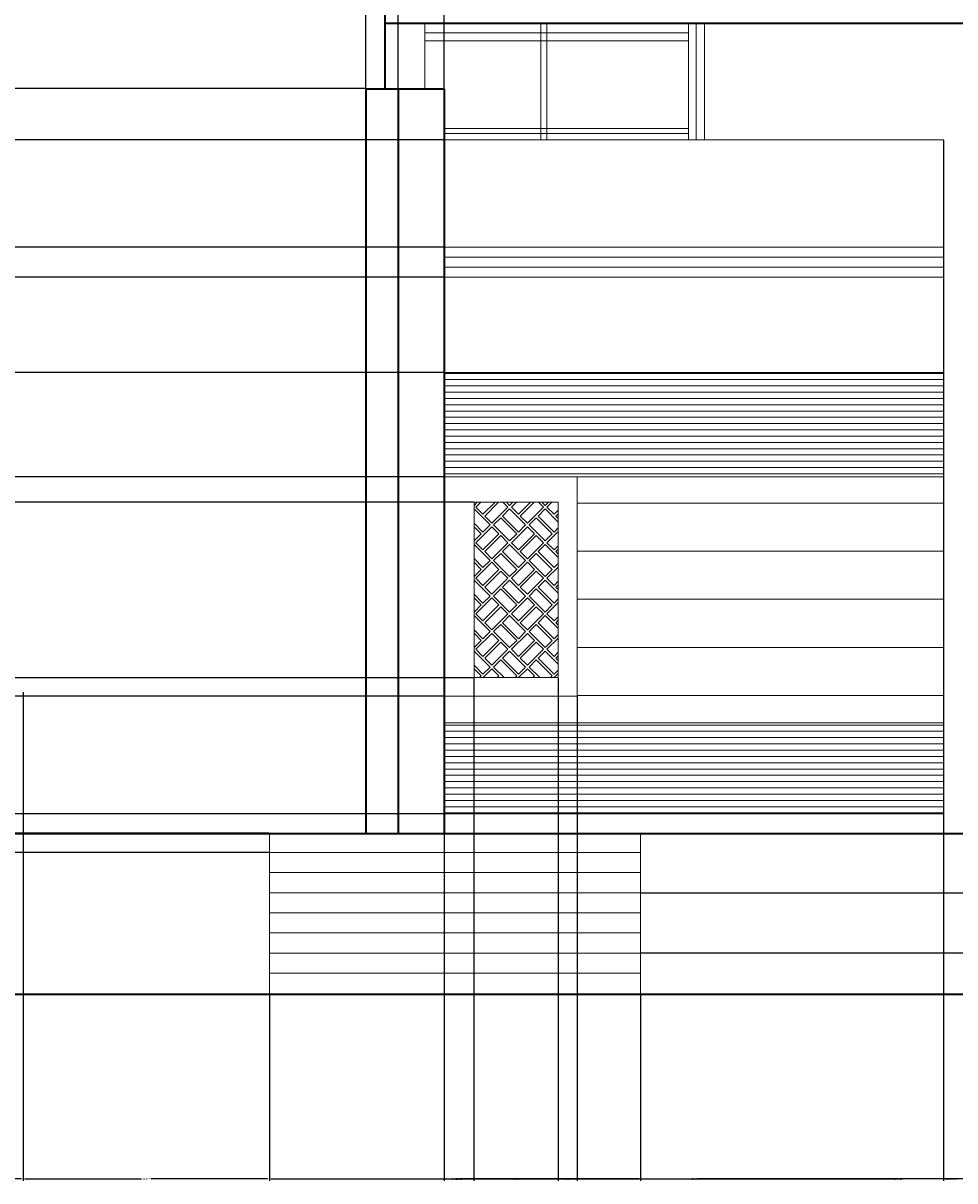
# Model space of a CAD drawing. Units: inches. Extents: x -7 to 391, y -12 to 303.
# Tile 3 of 5: x 222 to 315, y -12 to 103. Entities that reach past the tile are written whole.
import ezdxf

# ---------------------------------------------------------------- set-up
doc = ezdxf.new("R2010")
doc.units = ezdxf.units.IN
doc.header["$MEASUREMENT"] = 0
for name, color, linetype, lineweight in [('A-ANNO-DIMS', 2, 'Continuous', 18), ('A-DOOR', 3, 'Continuous', 18), ('A-ELEV', 7, 'Continuous', 35), ('A-ELEV-PATT', 8, 'Continuous', 13), ('A-FLOR-STRS', 2, 'Continuous', 18), ('A-GLAZ', 4, 'Continuous', 18)]:
    doc.layers.add(name, color=color, linetype=linetype, lineweight=lineweight)
doc.styles.get("Standard").update_dxf_attribs({"font": 'arial.ttf'})
doc.dimstyles.get("Standard").update_dxf_attribs({"dimtxt": 0.18, "dimasz": 0.18, "dimexe": 0.18, "dimexo": 0.0625, "dimgap": 0.09, "dimtad": 0, "dimtih": 1, "dimtoh": 1, "dimdec": 4, "dimzin": 0, "dimdsep": 46, "dimtxsty": 'Standard', "dimcen": 0.09, "dimadec": 0, "dimazin": 0, "dimtfac": 1, "dimtdec": 4, "dimtofl": 0, "dimtmove": 0, "dimatfit": 3, "dimfxl": 1, "dimtolj": 1, "dimtzin": 0, "dimarcsym": 0})

# ---------------------------------------------------------------- blocks, each defined once
blk = doc.blocks.new('*D1')
at = {"layer": 'A-ANNO-DIMS', "color": 0, "lineweight": -2, "transparency": 16777216}
for p, q in [((372.08, 122.18), (390.6, 122.18)), ((390.42, 122), (390.42, 64.44)), ((390.42, 6.53), (390.42, 64.08)), ((150.31, 6.35), (390.6, 6.35))]:
    blk.add_line(p, q, dxfattribs=at)
at = {"layer": 'A-ANNO-DIMS', "color": 0, "transparency": 16777216}
for points in [[(390.39, 122), (390.45, 122), (390.42, 122.18)], [(390.39, 6.53), (390.45, 6.53), (390.42, 6.35)]]:
    blk.add_solid(points, dxfattribs=at)
at = {"layer": 'Defpoints', "color": 0, "transparency": 16777216}
for p in [(372.02, 122.18), (390.42, 122.18), (150.24, 6.35)]:
    blk.add_point(p, dxfattribs=at)
at = {"layer": 'A-ANNO-DIMS', "color": 0, "transparency": 16777216, "insert": (390.42, 64.26), "char_height": 0.18, "attachment_point": 5}
blk.add_mtext('\\A1;115.83', dxfattribs=at)
blk = doc.blocks.new('*D37')
at = {"layer": 'A-ANNO-DIMS', "color": 0, "lineweight": -2, "transparency": 16777216}
for p, q in [((207.51, 38.39), (207.51, -12.23)), ((222.24, 36.39), (222.24, -12.23)), ((207.69, -12.05), (214.42, -12.05)), ((222.06, -12.05), (215.33, -12.05))]:
    blk.add_line(p, q, dxfattribs=at)
at = {"layer": 'A-ANNO-DIMS', "color": 0, "transparency": 16777216}
for points in [[(207.69, -12.02), (207.69, -12.08), (207.51, -12.05)], [(222.06, -12.02), (222.06, -12.08), (222.24, -12.05)]]:
    blk.add_solid(points, dxfattribs=at)
at = {"layer": 'Defpoints', "color": 0, "transparency": 16777216}
for p in [(207.51, 38.46), (222.24, 36.46), (222.24, -12.05)]:
    blk.add_point(p, dxfattribs=at)
at = {"layer": 'A-ANNO-DIMS', "color": 0, "transparency": 16777216, "insert": (214.88, -12.05), "char_height": 0.18, "attachment_point": 5}
blk.add_mtext('\\A1;14.734', dxfattribs=at)
blk = doc.blocks.new('*D38')
at = {"layer": 'A-ANNO-DIMS', "color": 0, "lineweight": -2, "transparency": 16777216}
for p, q in [((222.24, 36.39), (222.24, -12.23)), ((246.74, 6.28), (246.74, -12.23)), ((222.42, -12.05), (234.03, -12.05)), ((246.56, -12.05), (234.96, -12.05))]:
    blk.add_line(p, q, dxfattribs=at)
at = {"layer": 'A-ANNO-DIMS', "color": 0, "transparency": 16777216}
for points in [[(222.42, -12.02), (222.42, -12.08), (222.24, -12.05)], [(246.56, -12.02), (246.56, -12.08), (246.74, -12.05)]]:
    blk.add_solid(points, dxfattribs=at)
at = {"layer": 'Defpoints', "color": 0, "transparency": 16777216}
for p in [(222.24, 36.46), (246.74, 6.35), (246.74, -12.05)]:
    blk.add_point(p, dxfattribs=at)
at = {"layer": 'A-ANNO-DIMS', "color": 0, "transparency": 16777216, "insert": (234.49, -12.05), "char_height": 0.18, "attachment_point": 5}
blk.add_mtext('\\A1;24.497', dxfattribs=at)
blk = doc.blocks.new('*D39')
at = {"layer": 'A-ANNO-DIMS', "color": 0, "lineweight": -2, "transparency": 16777216}
for p, q in [((372.02, 154.28), (372.02, -12.23)), ((246.74, 6.28), (246.74, -12.23)), ((246.92, -12.05), (308.92, -12.05)), ((371.84, -12.05), (309.84, -12.05))]:
    blk.add_line(p, q, dxfattribs=at)
at = {"layer": 'A-ANNO-DIMS', "color": 0, "transparency": 16777216}
for points in [[(246.92, -12.02), (246.92, -12.08), (246.74, -12.05)], [(371.84, -12.02), (371.84, -12.08), (372.02, -12.05)]]:
    blk.add_solid(points, dxfattribs=at)
at = {"layer": 'Defpoints', "color": 0, "transparency": 16777216}
for p in [(372.02, 154.35), (246.74, 6.35), (372.02, -12.05)]:
    blk.add_point(p, dxfattribs=at)
at = {"layer": 'A-ANNO-DIMS', "color": 0, "transparency": 16777216, "insert": (309.38, -12.05), "char_height": 0.18, "attachment_point": 5}
blk.add_mtext('\\A1;125.28', dxfattribs=at)
blk = doc.blocks.new('*D40')
at = {"layer": 'A-ANNO-DIMS', "color": 0, "lineweight": -2, "transparency": 16777216}
for p, q in [((246.74, 6.28), (246.74, -12.23)), ((283.68, 6.28), (283.68, -12.23)), ((246.92, -12.05), (264.82, -12.05)), ((283.5, -12.05), (265.6, -12.05))]:
    blk.add_line(p, q, dxfattribs=at)
at = {"layer": 'A-ANNO-DIMS', "color": 0, "transparency": 16777216}
for points in [[(246.92, -12.02), (246.92, -12.08), (246.74, -12.05)], [(283.5, -12.02), (283.5, -12.08), (283.68, -12.05)]]:
    blk.add_solid(points, dxfattribs=at)
at = {"layer": 'Defpoints', "color": 0, "transparency": 16777216}
for p in [(246.74, 6.35), (283.68, 6.35), (283.68, -12.05)]:
    blk.add_point(p, dxfattribs=at)
at = {"layer": 'A-ANNO-DIMS', "color": 0, "transparency": 16777216, "insert": (265.21, -12.05), "char_height": 0.18, "attachment_point": 5}
blk.add_mtext('\\A1;36.94', dxfattribs=at)
blk = doc.blocks.new('*D41')
at = {"layer": 'A-ANNO-DIMS', "color": 0, "lineweight": -2, "transparency": 16777216}
for p, q in [((283.68, 6.28), (283.68, -12.23)), ((335.08, 6.28), (335.08, -12.23)), ((283.86, -12.05), (309.06, -12.05)), ((334.9, -12.05), (309.7, -12.05))]:
    blk.add_line(p, q, dxfattribs=at)
at = {"layer": 'A-ANNO-DIMS', "color": 0, "transparency": 16777216}
for points in [[(283.86, -12.02), (283.86, -12.08), (283.68, -12.05)], [(334.9, -12.02), (334.9, -12.08), (335.08, -12.05)]]:
    blk.add_solid(points, dxfattribs=at)
at = {"layer": 'Defpoints', "color": 0, "transparency": 16777216}
for p in [(283.68, 6.35), (335.08, 6.35), (335.08, -12.05)]:
    blk.add_point(p, dxfattribs=at)
at = {"layer": 'A-ANNO-DIMS', "color": 0, "transparency": 16777216, "insert": (309.38, -12.05), "char_height": 0.18, "attachment_point": 5}
blk.add_mtext('\\A1;51.4', dxfattribs=at)
blk = doc.blocks.new('*D43')
at = {"layer": 'A-ANNO-DIMS', "color": 0, "lineweight": -2, "transparency": 16777216}
for p, q in [((267.1, 37.78), (267.1, -12.23)), ((264.13, 35.95), (264.13, -12.23)), ((264.31, -12.05), (265.24, -12.05)), ((266.92, -12.05), (266, -12.05))]:
    blk.add_line(p, q, dxfattribs=at)
at = {"layer": 'A-ANNO-DIMS', "color": 0, "transparency": 16777216}
for points in [[(264.31, -12.02), (264.31, -12.08), (264.13, -12.05)], [(266.92, -12.02), (266.92, -12.08), (267.1, -12.05)]]:
    blk.add_solid(points, dxfattribs=at)
at = {"layer": 'Defpoints', "color": 0, "transparency": 16777216}
for p in [(267.1, 37.84), (264.13, 36.01), (267.1, -12.05)]:
    blk.add_point(p, dxfattribs=at)
at = {"layer": 'A-ANNO-DIMS', "color": 0, "transparency": 16777216, "insert": (265.62, -12.05), "char_height": 0.18, "attachment_point": 5}
blk.add_mtext('\\A1;2.971', dxfattribs=at)
blk = doc.blocks.new('*D44')
at = {"layer": 'A-ANNO-DIMS', "color": 0, "lineweight": -2, "transparency": 16777216}
for p, q in [((267.1, 37.78), (267.1, -12.23)), ((275.48, 37.78), (275.48, -12.23)), ((267.28, -12.05), (270.9, -12.05)), ((275.3, -12.05), (271.69, -12.05))]:
    blk.add_line(p, q, dxfattribs=at)
at = {"layer": 'A-ANNO-DIMS', "color": 0, "transparency": 16777216}
for points in [[(267.28, -12.02), (267.28, -12.08), (267.1, -12.05)], [(275.3, -12.02), (275.3, -12.08), (275.48, -12.05)]]:
    blk.add_solid(points, dxfattribs=at)
at = {"layer": 'Defpoints', "color": 0, "transparency": 16777216}
for p in [(267.1, 37.84), (275.48, 37.84), (275.48, -12.05)]:
    blk.add_point(p, dxfattribs=at)
at = {"layer": 'A-ANNO-DIMS', "color": 0, "transparency": 16777216, "insert": (271.29, -12.05), "char_height": 0.18, "attachment_point": 5}
blk.add_mtext('\\A1;8.377', dxfattribs=at)
blk = doc.blocks.new('*D45')
at = {"layer": 'A-ANNO-DIMS', "color": 0, "lineweight": -2, "transparency": 16777216}
for p, q in [((275.48, 37.78), (275.48, -12.23)), ((277.36, 35.95), (277.36, -12.23)), ((275.66, -12.05), (276.1, -12.05)), ((277.18, -12.05), (276.74, -12.05))]:
    blk.add_line(p, q, dxfattribs=at)
at = {"layer": 'A-ANNO-DIMS', "color": 0, "transparency": 16777216}
for points in [[(275.66, -12.02), (275.66, -12.08), (275.48, -12.05)], [(277.18, -12.02), (277.18, -12.08), (277.36, -12.05)]]:
    blk.add_solid(points, dxfattribs=at)
at = {"layer": 'Defpoints', "color": 0, "transparency": 16777216}
for p in [(275.48, 37.84), (277.36, 36.01), (277.36, -12.05)]:
    blk.add_point(p, dxfattribs=at)
at = {"layer": 'A-ANNO-DIMS', "color": 0, "transparency": 16777216, "insert": (276.42, -12.05), "char_height": 0.18, "attachment_point": 5}
blk.add_mtext('\\A1;1.88', dxfattribs=at)
blk = doc.blocks.new('*D46')
at = {"layer": 'A-ANNO-DIMS', "color": 0, "lineweight": -2, "transparency": 16777216}
for p, q in [((256.34, 96.52), (256.34, 303.01)), ((259.55, 96.52), (259.55, 303.01)), ((256.52, 302.83), (257.55, 302.83)), ((259.37, 302.83), (258.34, 302.83))]:
    blk.add_line(p, q, dxfattribs=at)
at = {"layer": 'A-ANNO-DIMS', "color": 0, "transparency": 16777216}
for points in [[(256.52, 302.86), (256.52, 302.8), (256.34, 302.83)], [(259.37, 302.86), (259.37, 302.8), (259.55, 302.83)]]:
    blk.add_solid(points, dxfattribs=at)
at = {"layer": 'Defpoints', "color": 0, "transparency": 16777216}
for p in [(259.55, 302.83), (256.34, 96.46), (259.55, 96.46)]:
    blk.add_point(p, dxfattribs=at)
at = {"layer": 'A-ANNO-DIMS', "color": 0, "transparency": 16777216, "insert": (257.95, 302.83), "char_height": 0.18, "attachment_point": 5}
blk.add_mtext('\\A1;3.217', dxfattribs=at)
blk = doc.blocks.new('*D47')
at = {"layer": 'A-ANNO-DIMS', "color": 0, "lineweight": -2, "transparency": 16777216}
for p, q in [((259.55, 96.52), (259.55, 303.01)), ((264.13, 96.52), (264.13, 303.01)), ((259.73, 302.83), (261.45, 302.83)), ((263.95, 302.83), (262.24, 302.83))]:
    blk.add_line(p, q, dxfattribs=at)
at = {"layer": 'A-ANNO-DIMS', "color": 0, "transparency": 16777216}
for points in [[(259.73, 302.86), (259.73, 302.8), (259.55, 302.83)], [(263.95, 302.86), (263.95, 302.8), (264.13, 302.83)]]:
    blk.add_solid(points, dxfattribs=at)
at = {"layer": 'Defpoints', "color": 0, "transparency": 16777216}
for p in [(264.13, 302.83), (259.55, 96.46), (264.13, 96.46)]:
    blk.add_point(p, dxfattribs=at)
at = {"layer": 'A-ANNO-DIMS', "color": 0, "transparency": 16777216, "insert": (261.84, 302.83), "char_height": 0.18, "attachment_point": 5}
blk.add_mtext('\\A1;4.579', dxfattribs=at)
blk = doc.blocks.new('*D48')
at = {"layer": 'A-ANNO-DIMS', "color": 0, "lineweight": -2, "transparency": 16777216}
for p, q in [((264.13, 91.3), (264.13, -12.23)), ((313.81, 91.3), (313.81, -12.23)), ((264.31, -12.05), (288.57, -12.05)), ((313.63, -12.05), (289.37, -12.05))]:
    blk.add_line(p, q, dxfattribs=at)
at = {"layer": 'A-ANNO-DIMS', "color": 0, "transparency": 16777216}
for points in [[(264.31, -12.02), (264.31, -12.08), (264.13, -12.05)], [(313.63, -12.02), (313.63, -12.08), (313.81, -12.05)]]:
    blk.add_solid(points, dxfattribs=at)
at = {"layer": 'Defpoints', "color": 0, "transparency": 16777216}
for p in [(264.13, 91.37), (313.81, 91.37), (313.81, -12.05)]:
    blk.add_point(p, dxfattribs=at)
at = {"layer": 'A-ANNO-DIMS', "color": 0, "transparency": 16777216, "insert": (288.97, -12.05), "char_height": 0.18, "attachment_point": 5}
blk.add_mtext('\\A1;49.68', dxfattribs=at)
blk = doc.blocks.new('*D49')
at = {"layer": 'A-ANNO-DIMS', "color": 0, "lineweight": -2, "transparency": 16777216}
for p, q in [((313.81, 91.3), (313.81, -12.23)), ((316.08, 91.3), (316.08, -12.23)), ((313.99, -12.05), (314.62, -12.05)), ((315.9, -12.05), (315.27, -12.05))]:
    blk.add_line(p, q, dxfattribs=at)
at = {"layer": 'A-ANNO-DIMS', "color": 0, "transparency": 16777216}
for points in [[(313.99, -12.02), (313.99, -12.08), (313.81, -12.05)], [(315.9, -12.02), (315.9, -12.08), (316.08, -12.05)]]:
    blk.add_solid(points, dxfattribs=at)
at = {"layer": 'Defpoints', "color": 0, "transparency": 16777216}
for p in [(313.81, 91.37), (316.08, 91.37), (316.08, -12.05)]:
    blk.add_point(p, dxfattribs=at)
at = {"layer": 'A-ANNO-DIMS', "color": 0, "transparency": 16777216, "insert": (314.94, -12.05), "char_height": 0.18, "attachment_point": 5}
blk.add_mtext('\\A1;2.27', dxfattribs=at)
blk = doc.blocks.new('*D53')
at = {"layer": 'A-ANNO-DIMS', "color": 0, "lineweight": -2, "transparency": 16777216}
for p, q in [((256.34, 96.52), (256.34, 303.01)), ((258.27, 103.04), (258.27, 303.01)), ((256.52, 302.83), (256.92, 302.83)), ((258.09, 302.83), (257.69, 302.83))]:
    blk.add_line(p, q, dxfattribs=at)
at = {"layer": 'A-ANNO-DIMS', "color": 0, "transparency": 16777216}
for points in [[(256.52, 302.86), (256.52, 302.8), (256.34, 302.83)], [(258.09, 302.86), (258.09, 302.8), (258.27, 302.83)]]:
    blk.add_solid(points, dxfattribs=at)
at = {"layer": 'Defpoints', "color": 0, "transparency": 16777216}
for p in [(258.27, 302.83), (258.27, 102.98), (256.34, 96.46)]:
    blk.add_point(p, dxfattribs=at)
at = {"layer": 'A-ANNO-DIMS', "color": 0, "transparency": 16777216, "insert": (257.3, 302.83), "char_height": 0.18, "attachment_point": 5}
blk.add_mtext('\\A1;1.933', dxfattribs=at)
blk = doc.blocks.new('*D64')
at = {"layer": 'A-ANNO-DIMS', "color": 0, "lineweight": -2, "transparency": 16777216}
for p, q in [((264.07, 24.3), (-6.56, 24.3)), ((-6.38, 24.12), (-6.38, 23.5)), ((-6.38, 22.53), (-6.38, 23.14)), ((246.68, 22.35), (-6.56, 22.35))]:
    blk.add_line(p, q, dxfattribs=at)
at = {"layer": 'A-ANNO-DIMS', "color": 0, "transparency": 16777216}
for points in [[(-6.41, 24.12), (-6.35, 24.12), (-6.38, 24.3)], [(-6.41, 22.53), (-6.35, 22.53), (-6.38, 22.35)]]:
    blk.add_solid(points, dxfattribs=at)
at = {"layer": 'Defpoints', "color": 0, "transparency": 16777216}
for p in [(-6.38, 24.3), (264.13, 24.3), (246.74, 22.35)]:
    blk.add_point(p, dxfattribs=at)
at = {"layer": 'A-ANNO-DIMS', "color": 0, "transparency": 16777216, "insert": (-6.38, 23.32), "char_height": 0.18, "attachment_point": 5}
blk.add_mtext('\\A1;1.952', dxfattribs=at)
blk = doc.blocks.new('*D65')
at = {"layer": 'A-ANNO-DIMS', "color": 0, "lineweight": -2, "transparency": 16777216}
for p, q in [((264.07, 36.01), (-6.56, 36.01)), ((-6.38, 35.83), (-6.38, 30.34)), ((-6.38, 24.48), (-6.38, 29.97)), ((264.07, 24.3), (-6.56, 24.3))]:
    blk.add_line(p, q, dxfattribs=at)
at = {"layer": 'A-ANNO-DIMS', "color": 0, "transparency": 16777216}
for points in [[(-6.41, 35.83), (-6.35, 35.83), (-6.38, 36.01)], [(-6.41, 24.48), (-6.35, 24.48), (-6.38, 24.3)]]:
    blk.add_solid(points, dxfattribs=at)
at = {"layer": 'Defpoints', "color": 0, "transparency": 16777216}
for p in [(-6.38, 36.01), (264.13, 36.01), (264.13, 24.3)]:
    blk.add_point(p, dxfattribs=at)
at = {"layer": 'A-ANNO-DIMS', "color": 0, "transparency": 16777216, "insert": (-6.38, 30.16), "char_height": 0.18, "attachment_point": 5}
blk.add_mtext('\\A1;11.716', dxfattribs=at)
blk = doc.blocks.new('*D66')
at = {"layer": 'A-ANNO-DIMS', "color": 0, "lineweight": -2, "transparency": 16777216}
for p, q in [((264.07, 57.83), (-6.56, 57.83)), ((-6.38, 57.65), (-6.38, 47.1)), ((-6.38, 36.19), (-6.38, 46.74)), ((264.07, 36.01), (-6.56, 36.01))]:
    blk.add_line(p, q, dxfattribs=at)
at = {"layer": 'A-ANNO-DIMS', "color": 0, "transparency": 16777216}
for points in [[(-6.41, 57.65), (-6.35, 57.65), (-6.38, 57.83)], [(-6.41, 36.19), (-6.35, 36.19), (-6.38, 36.01)]]:
    blk.add_solid(points, dxfattribs=at)
at = {"layer": 'Defpoints', "color": 0, "transparency": 16777216}
for p in [(-6.38, 57.83), (264.13, 57.83), (264.13, 36.01)]:
    blk.add_point(p, dxfattribs=at)
at = {"layer": 'A-ANNO-DIMS', "color": 0, "transparency": 16777216, "insert": (-6.38, 46.92), "char_height": 0.18, "attachment_point": 5}
blk.add_mtext('\\A1;21.82', dxfattribs=at)
blk = doc.blocks.new('*D67')
at = {"layer": 'A-ANNO-DIMS', "color": 0, "lineweight": -2, "transparency": 16777216}
for p, q in [((264.07, 68.22), (-6.56, 68.22)), ((-6.38, 68.04), (-6.38, 63.21)), ((-6.38, 58.01), (-6.38, 62.84)), ((264.07, 57.83), (-6.56, 57.83))]:
    blk.add_line(p, q, dxfattribs=at)
at = {"layer": 'A-ANNO-DIMS', "color": 0, "transparency": 16777216}
for points in [[(-6.41, 68.04), (-6.35, 68.04), (-6.38, 68.22)], [(-6.41, 58.01), (-6.35, 58.01), (-6.38, 57.83)]]:
    blk.add_solid(points, dxfattribs=at)
at = {"layer": 'Defpoints', "color": 0, "transparency": 16777216}
for p in [(-6.38, 68.22), (264.13, 68.22), (264.13, 57.83)]:
    blk.add_point(p, dxfattribs=at)
at = {"layer": 'A-ANNO-DIMS', "color": 0, "transparency": 16777216, "insert": (-6.38, 63.03), "char_height": 0.18, "attachment_point": 5}
blk.add_mtext('\\A1;10.388', dxfattribs=at)
blk = doc.blocks.new('*D68')
at = {"layer": 'A-ANNO-DIMS', "color": 0, "lineweight": -2, "transparency": 16777216}
for p, q in [((264.07, 77.69), (-6.56, 77.69)), ((-6.38, 77.51), (-6.38, 73.14)), ((-6.38, 68.4), (-6.38, 72.77)), ((264.07, 68.22), (-6.56, 68.22))]:
    blk.add_line(p, q, dxfattribs=at)
at = {"layer": 'A-ANNO-DIMS', "color": 0, "transparency": 16777216}
for points in [[(-6.41, 77.51), (-6.35, 77.51), (-6.38, 77.69)], [(-6.41, 68.4), (-6.35, 68.4), (-6.38, 68.22)]]:
    blk.add_solid(points, dxfattribs=at)
at = {"layer": 'Defpoints', "color": 0, "transparency": 16777216}
for p in [(-6.38, 77.69), (264.13, 77.69), (264.13, 68.22)]:
    blk.add_point(p, dxfattribs=at)
at = {"layer": 'A-ANNO-DIMS', "color": 0, "transparency": 16777216, "insert": (-6.38, 72.96), "char_height": 0.18, "attachment_point": 5}
blk.add_mtext('\\A1;9.474', dxfattribs=at)
blk = doc.blocks.new('*D69')
at = {"layer": 'A-ANNO-DIMS', "color": 0, "lineweight": -2, "transparency": 16777216}
for p, q in [((264.07, 80.69), (-6.56, 80.69)), ((-6.38, 80.51), (-6.38, 79.38)), ((-6.38, 77.87), (-6.38, 79.01)), ((264.07, 77.69), (-6.56, 77.69))]:
    blk.add_line(p, q, dxfattribs=at)
at = {"layer": 'A-ANNO-DIMS', "color": 0, "transparency": 16777216}
for points in [[(-6.41, 80.51), (-6.35, 80.51), (-6.38, 80.69)], [(-6.41, 77.87), (-6.35, 77.87), (-6.38, 77.69)]]:
    blk.add_solid(points, dxfattribs=at)
at = {"layer": 'Defpoints', "color": 0, "transparency": 16777216}
for p in [(-6.38, 80.69), (264.13, 80.69), (264.13, 77.69)]:
    blk.add_point(p, dxfattribs=at)
at = {"layer": 'A-ANNO-DIMS', "color": 0, "transparency": 16777216, "insert": (-6.38, 79.19), "char_height": 0.18, "attachment_point": 5}
blk.add_mtext('\\A1;3', dxfattribs=at)
blk = doc.blocks.new('*D70')
at = {"layer": 'A-ANNO-DIMS', "color": 0, "lineweight": -2, "transparency": 16777216}
for p, q in [((264.07, 91.37), (-6.56, 91.37)), ((-6.38, 91.19), (-6.38, 86.21)), ((-6.38, 80.87), (-6.38, 85.85)), ((264.07, 80.69), (-6.56, 80.69))]:
    blk.add_line(p, q, dxfattribs=at)
at = {"layer": 'A-ANNO-DIMS', "color": 0, "transparency": 16777216}
for points in [[(-6.41, 91.19), (-6.35, 91.19), (-6.38, 91.37)], [(-6.41, 80.87), (-6.35, 80.87), (-6.38, 80.69)]]:
    blk.add_solid(points, dxfattribs=at)
at = {"layer": 'Defpoints', "color": 0, "transparency": 16777216}
for p in [(-6.38, 91.37), (264.13, 91.37), (264.13, 80.69)]:
    blk.add_point(p, dxfattribs=at)
at = {"layer": 'A-ANNO-DIMS', "color": 0, "transparency": 16777216, "insert": (-6.38, 86.03), "char_height": 0.18, "attachment_point": 5}
blk.add_mtext('\\A1;10.672', dxfattribs=at)
blk = doc.blocks.new('*D71')
at = {"layer": 'A-ANNO-DIMS', "color": 0, "lineweight": -2, "transparency": 16777216}
for p, q in [((256.28, 96.46), (-6.56, 96.46)), ((-6.38, 96.28), (-6.38, 94.09)), ((-6.38, 91.55), (-6.38, 93.73)), ((264.07, 91.37), (-6.56, 91.37))]:
    blk.add_line(p, q, dxfattribs=at)
at = {"layer": 'A-ANNO-DIMS', "color": 0, "transparency": 16777216}
for points in [[(-6.41, 96.28), (-6.35, 96.28), (-6.38, 96.46)], [(-6.41, 91.55), (-6.35, 91.55), (-6.38, 91.37)]]:
    blk.add_solid(points, dxfattribs=at)
at = {"layer": 'Defpoints', "color": 0, "transparency": 16777216}
for p in [(-6.38, 96.46), (256.34, 96.46), (264.13, 91.37)]:
    blk.add_point(p, dxfattribs=at)
at = {"layer": 'A-ANNO-DIMS', "color": 0, "transparency": 16777216, "insert": (-6.38, 93.91), "char_height": 0.18, "attachment_point": 5}
blk.add_mtext('\\A1;5.09', dxfattribs=at)
blk = doc.blocks.new('*D72')
at = {"layer": 'A-ANNO-DIMS', "color": 0, "lineweight": -2, "transparency": 16777216}
for p, q in [((267.04, 55.3), (-6.56, 55.3)), ((-6.38, 55.12), (-6.38, 46.75)), ((-6.38, 38.02), (-6.38, 46.39)), ((267.04, 37.84), (-6.56, 37.84))]:
    blk.add_line(p, q, dxfattribs=at)
at = {"layer": 'A-ANNO-DIMS', "color": 0, "transparency": 16777216}
for points in [[(-6.41, 55.12), (-6.35, 55.12), (-6.38, 55.3)], [(-6.41, 38.02), (-6.35, 38.02), (-6.38, 37.84)]]:
    blk.add_solid(points, dxfattribs=at)
at = {"layer": 'Defpoints', "color": 0, "transparency": 16777216}
for p in [(-6.38, 55.3), (267.1, 55.3), (267.1, 37.84)]:
    blk.add_point(p, dxfattribs=at)
at = {"layer": 'A-ANNO-DIMS', "color": 0, "transparency": 16777216, "insert": (-6.38, 46.57), "char_height": 0.18, "attachment_point": 5}
blk.add_mtext('\\A1;17.455', dxfattribs=at)
blk = doc.blocks.new('*D73')
at = {"layer": 'A-ANNO-DIMS', "color": 0, "lineweight": -2, "transparency": 16777216}
for p, q in [((246.68, 22.35), (-6.56, 22.35)), ((-6.38, 22.17), (-6.38, 21.57)), ((-6.38, 20.62), (-6.38, 21.21)), ((246.68, 20.44), (-6.56, 20.44))]:
    blk.add_line(p, q, dxfattribs=at)
at = {"layer": 'A-ANNO-DIMS', "color": 0, "transparency": 16777216}
for points in [[(-6.41, 22.17), (-6.35, 22.17), (-6.38, 22.35)], [(-6.41, 20.62), (-6.35, 20.62), (-6.38, 20.44)]]:
    blk.add_solid(points, dxfattribs=at)
at = {"layer": 'Defpoints', "color": 0, "transparency": 16777216}
for p in [(-6.38, 22.35), (246.74, 22.35), (246.74, 20.44)]:
    blk.add_point(p, dxfattribs=at)
at = {"layer": 'A-ANNO-DIMS', "color": 0, "transparency": 16777216, "insert": (-6.38, 21.39), "char_height": 0.18, "attachment_point": 5}
blk.add_mtext('\\A1;1.91', dxfattribs=at)
blk = doc.blocks.new('*D74')
at = {"layer": 'A-ANNO-DIMS', "color": 0, "lineweight": -2, "transparency": 16777216}
for p, q in [((283.74, 10.44), (390.6, 10.44)), ((390.42, 10.26), (390.42, 8.57)), ((390.42, 6.53), (390.42, 8.21)), ((283.74, 6.35), (390.6, 6.35))]:
    blk.add_line(p, q, dxfattribs=at)
at = {"layer": 'A-ANNO-DIMS', "color": 0, "transparency": 16777216}
for points in [[(390.39, 10.26), (390.45, 10.26), (390.42, 10.44)], [(390.39, 6.53), (390.45, 6.53), (390.42, 6.35)]]:
    blk.add_solid(points, dxfattribs=at)
at = {"layer": 'Defpoints', "color": 0, "transparency": 16777216}
for p in [(283.68, 10.44), (390.42, 10.44), (283.68, 6.35)]:
    blk.add_point(p, dxfattribs=at)
at = {"layer": 'A-ANNO-DIMS', "color": 0, "transparency": 16777216, "insert": (390.42, 8.39), "char_height": 0.18, "attachment_point": 5}
blk.add_mtext('\\A1;4.094', dxfattribs=at)
blk = doc.blocks.new('*D75')
at = {"layer": 'A-ANNO-DIMS', "color": 0, "lineweight": -2, "transparency": 16777216}
for p, q in [((283.74, 16.44), (390.6, 16.44)), ((390.42, 16.26), (390.42, 13.62)), ((390.42, 10.62), (390.42, 13.26)), ((283.74, 10.44), (390.6, 10.44))]:
    blk.add_line(p, q, dxfattribs=at)
at = {"layer": 'A-ANNO-DIMS', "color": 0, "transparency": 16777216}
for points in [[(390.39, 16.26), (390.45, 16.26), (390.42, 16.44)], [(390.39, 10.62), (390.45, 10.62), (390.42, 10.44)]]:
    blk.add_solid(points, dxfattribs=at)
at = {"layer": 'Defpoints', "color": 0, "transparency": 16777216}
for p in [(283.68, 16.44), (390.42, 16.44), (283.68, 10.44)]:
    blk.add_point(p, dxfattribs=at)
at = {"layer": 'A-ANNO-DIMS', "color": 0, "transparency": 16777216, "insert": (390.42, 13.44), "char_height": 0.18, "attachment_point": 5}
blk.add_mtext('\\A1;6', dxfattribs=at)
blk = doc.blocks.new('*D76')
at = {"layer": 'A-ANNO-DIMS', "color": 0, "lineweight": -2, "transparency": 16777216}
for p, q in [((283.74, 22.35), (390.6, 22.35)), ((390.42, 22.17), (390.42, 19.57)), ((390.42, 16.62), (390.42, 19.21)), ((283.74, 16.44), (390.6, 16.44))]:
    blk.add_line(p, q, dxfattribs=at)
at = {"layer": 'A-ANNO-DIMS', "color": 0, "transparency": 16777216}
for points in [[(390.39, 22.17), (390.45, 22.17), (390.42, 22.35)], [(390.39, 16.62), (390.45, 16.62), (390.42, 16.44)]]:
    blk.add_solid(points, dxfattribs=at)
at = {"layer": 'Defpoints', "color": 0, "transparency": 16777216}
for p in [(283.68, 22.35), (390.42, 22.35), (283.68, 16.44)]:
    blk.add_point(p, dxfattribs=at)
at = {"layer": 'A-ANNO-DIMS', "color": 0, "transparency": 16777216, "insert": (390.42, 19.39), "char_height": 0.18, "attachment_point": 5}
blk.add_mtext('\\A1;5.906', dxfattribs=at)

msp = doc.modelspace()

# ---------------------------------------------------------------- hatches: boundary and pattern name
at = {"layer": 'A-ELEV-PATT'}
h = msp.add_hatch(dxfattribs=at)
h.set_pattern_fill('ANSI31', color=256, scale=5, angle=135)
h.paths.add_polyline_path([(313.8105, 33.3417), (264.1332, 33.3417), (264.1332, 24.2974), (313.8105, 24.2974)])
h.paths.add_polyline_path([(362.5506, 32.9858), (316.076, 32.9858), (316.076, 24.2974), (362.5506, 24.2974)])
h.paths.add_polyline_path([(362.5506, 68.2193), (316.076, 68.2193), (316.076, 57.8315), (329.3009, 57.8315), (362.5506, 57.8315)])
h.paths.add_polyline_path([(313.8105, 68.2193), (264.1332, 68.2193), (264.1332, 57.8315), (313.8105, 57.8315)])
h = msp.add_hatch(dxfattribs=at)
h.set_pattern_fill('2X2µØ×©', color=256, scale=5, angle=135)
h.set_pattern_definition([(135, (0, 0), (-3.535534, 2e-16), [2.25, -0.25, 1, -0.25, 1, -0.25]), (135, (-0.707, -0.707), (-3.535534, 2e-16), [2.25, -2.75]), (135, (-0.884, -0.884), (-3.535534, 2e-16), [2.25, -2.75]), (135, (-1.591, -1.591), (-3.535534, 2e-16), [2.25, -0.25, 1, -0.25, 1, -0.25]), (225, (0, 0), (-4e-16, -3.535534), [1, -0.25, 1, -0.25, 2.25, -0.25]), (225, (-1.591, 1.591), (-4e-16, -3.535534), [1, -0.25, 1, -0.25, 2.25, -0.25]), (225, (-2.4749, 2.4749), (-4e-16, -3.535534), [2.25, -2.75]), (225, (-2.6517, 2.6517), (-4e-16, -3.535534), [2.25, -2.75])])
h.paths.add_polyline_path([(275.4815, 55.2969), (267.1041, 55.2969), (267.1041, 37.8416), (275.4815, 37.8416)])
h.paths.add_polyline_path([(327.4242, 55.2969), (319.0469, 55.2969), (319.0469, 37.8416), (327.4242, 37.8416)])

# ---------------------------------------------------------------- linework, layer by layer
at = {"layer": 'A-DOOR'}
for p, q in [((264.1332, 80.6934), (313.8105, 80.6934)), ((264.1332, 79.6934), (313.8105, 79.6934)), ((264.1332, 78.6934), (313.8105, 78.6934)), ((264.1332, 77.6934), (313.8105, 77.6934)), ((264.1332, 68.2193), (313.8105, 68.2193)), ((264.1332, 57.8315), (313.8105, 57.8315)), ((277.3582, 55.2077), (313.8105, 55.2077)), ((277.3582, 50.4241), (313.8105, 50.4241)), ((277.3582, 45.6405), (313.8105, 45.6405)), ((277.3582, 40.8569), (313.8105, 40.8569)), ((277.3582, 36.0733), (313.8105, 36.0733)), ((264.1332, 33.3417), (313.8105, 33.3417))]:
    msp.add_line(p, q, dxfattribs=at)
for points in [[(264.1332, 91.3657), (313.8105, 91.3657), (313.8105, 24.2974), (264.1332, 24.2974)], [(264.1332, 57.8315), (277.3582, 57.8315), (277.3582, 36.0134), (264.1332, 36.0134)], [(267.1041, 55.2969), (275.4815, 55.2969), (275.4815, 37.8416), (267.1041, 37.8416)]]:
    msp.add_lwpolyline(points, close=True, dxfattribs=at)
at = {"layer": 'A-ELEV'}
for p, q in [((258.2707, 96.456), (258.2707, 122.1767)), ((258.2707, 102.9762), (368.0993, 102.9762)), ((256.3377, 96.456), (264.1332, 96.456)), ((256.3377, 96.456), (256.3377, 22.3452)), ((259.5545, 96.456), (259.5545, 22.3452)), ((264.1332, 96.456), (264.1332, 22.3452)), ((12.0212, 22.3452), (372.0212, 22.3452)), ((12.0212, 6.3452), (372.0212, 6.3452))]:
    msp.add_line(p, q, dxfattribs=at)
at = {"layer": 'A-FLOR-STRS'}
for p, q in [((246.7395, 22.3452), (246.7395, 6.3452)), ((283.6807, 22.3452), (283.6807, 6.3452)), ((283.6807, 20.4396), (246.7395, 20.4396)), ((283.6807, 18.4396), (246.7395, 18.4396)), ((283.6807, 16.4396), (246.7395, 16.4396)), ((283.6807, 16.4396), (335.0799, 16.4396)), ((283.6807, 14.4396), (246.7395, 14.4396)), ((283.6807, 12.4396), (246.7395, 12.4396)), ((283.6807, 10.4396), (246.7395, 10.4396)), ((283.6807, 10.4396), (335.0799, 10.4396)), ((283.6807, 8.4396), (246.7395, 8.4396))]:
    msp.add_line(p, q, dxfattribs=at)
at = {"layer": 'A-GLAZ'}
for p, q in [((259.5545, 96.456), (259.5545, 102.9762)), ((262.2191, 96.456), (262.2191, 102.9762)), ((273.7532, 102.9762), (273.7532, 91.3657)), ((274.3484, 102.9762), (274.3484, 91.3657)), ((288.4588, 102.9762), (288.4588, 91.3657)), ((289.2213, 102.9762), (289.2213, 91.3657)), ((290.0289, 102.9762), (290.0289, 91.3657)), ((262.2191, 101.9983), (288.4588, 101.9983)), ((262.2191, 101.2108), (288.4588, 101.2108)), ((264.1332, 92.5065), (288.4588, 92.5065)), ((264.1332, 91.9913), (288.4588, 91.9913))]:
    msp.add_line(p, q, dxfattribs=at)

# ---------------------------------------------------------------- dimensions: what is measured, and where the dimension line sits
at = {"layer": 'A-ANNO-DIMS'}
for base, p1, p2, override, picture, middle in [((259.5545, 302.832), (256.3377, 96.456), (259.5545, 96.456), {"dimdec": 3, "dimlfac": 1, "dimrnd": 0, "dimzin": 0, "dimdsep": 46, "dimlunit": 2}, '*D46', (257.9461, 302.832)), ((258.2707, 302.832), (256.3377, 96.456), (258.2707, 102.9762), {"dimdec": 3, "dimlfac": 1, "dimrnd": 0, "dimzin": 0, "dimdsep": 46, "dimlunit": 2}, '*D53', (257.3042, 302.832)), ((264.1332, 302.832), (259.5545, 96.456), (264.1332, 96.456), {"dimdec": 3, "dimlfac": 1, "dimrnd": 0, "dimzin": 0, "dimdsep": 46, "dimlunit": 2}, '*D47', (261.8439, 302.832)), ((372.0212, -12.0548), (246.7395, 6.3452), (372.0212, 154.3452), {"dimdec": 2, "dimlfac": 1, "dimrnd": 0, "dimzin": 0, "dimdsep": 46, "dimlunit": 2}, '*D39', (309.3803, -12.0548)), ((313.8105, -12.0548), (264.1332, 91.3657), (313.8105, 91.3657), {"dimdec": 2, "dimlfac": 1, "dimrnd": 0, "dimzin": 0, "dimdsep": 46, "dimlunit": 2}, '*D48', (288.9719, -12.0548)), ((316.076, -12.0548), (313.8105, 91.3657), (316.076, 91.3657), {"dimdec": 2, "dimlfac": 1, "dimrnd": 0, "dimzin": 0, "dimdsep": 46, "dimlunit": 2}, '*D49', (314.9432, -12.0548)), ((222.2426, -12.0548), (207.5087, 38.456), (222.2426, 36.456), {"dimdec": 3, "dimlfac": 1, "dimrnd": 0, "dimzin": 0, "dimdsep": 46, "dimlunit": 2}, '*D37', (214.8756, -12.0548)), ((267.1041, -12.0548), (264.1332, 36.0134), (267.1041, 37.8416), {"dimdec": 3, "dimlfac": 1, "dimrnd": 0, "dimzin": 0, "dimdsep": 46, "dimlunit": 2}, '*D43', (265.6187, -12.0548)), ((275.4815, -12.0548), (267.1041, 37.8416), (275.4815, 37.8416), {"dimdec": 3, "dimlfac": 1, "dimrnd": 0, "dimzin": 0, "dimdsep": 46, "dimlunit": 2}, '*D44', (271.2928, -12.0548)), ((277.3582, -12.0548), (275.4815, 37.8416), (277.3582, 36.0134), {"dimdec": 2, "dimlfac": 1, "dimrnd": 0, "dimzin": 0, "dimdsep": 46, "dimlunit": 2}, '*D45', (276.4198, -12.0548)), ((246.7395, -12.0548), (222.2426, 36.456), (246.7395, 6.3452), {"dimdec": 3, "dimlfac": 1, "dimrnd": 0, "dimzin": 0, "dimdsep": 46, "dimlunit": 2}, '*D38', (234.491, -12.0548)), ((283.6807, -12.0548), (246.7395, 6.3452), (283.6807, 6.3452), {"dimdec": 2, "dimlfac": 1, "dimrnd": 0, "dimzin": 0, "dimdsep": 46, "dimlunit": 2}, '*D40', (265.2101, -12.0548)), ((335.0799, -12.0548), (283.6807, 6.3452), (335.0799, 6.3452), {"dimdec": 1, "dimlfac": 1, "dimrnd": 0, "dimzin": 0, "dimdsep": 46, "dimlunit": 2}, '*D41', (309.3803, -12.0548))]:
    dim = msp.add_linear_dim(base=base, p1=p1, p2=p2, dimstyle='Standard', override=override, dxfattribs=at)
    dim.commit()
    dim.dimension.update_dxf_attribs({"geometry": picture, "text_midpoint": middle})
for base, p1, p2, override, picture, middle in [((390.4212, 122.1767), (150.2426, 6.3452), (372.0212, 122.1767), {"dimdec": 2, "dimlfac": 1, "dimrnd": 0, "dimzin": 0, "dimdsep": 46, "dimlunit": 2}, '*D1', (390.4212, 64.261)), ((-6.3788, 96.456), (264.1332, 91.3657), (256.3377, 96.456), {"dimdec": 2, "dimlfac": 1, "dimrnd": 0, "dimzin": 0, "dimdsep": 46, "dimlunit": 2}, '*D71', (-6.3788, 93.9109)), ((-6.3788, 91.3657), (264.1332, 80.6934), (264.1332, 91.3657), {"dimdec": 3, "dimlfac": 1, "dimrnd": 0, "dimzin": 0, "dimdsep": 46, "dimlunit": 2}, '*D70', (-6.3788, 86.0296)), ((-6.3788, 80.6934), (264.1332, 77.6934), (264.1332, 80.6934), {"dimdec": 0, "dimlfac": 1, "dimrnd": 0, "dimzin": 0, "dimdsep": 46, "dimlunit": 2}, '*D69', (-6.3788, 79.1934)), ((-6.3788, 77.6934), (264.1332, 68.2193), (264.1332, 77.6934), {"dimdec": 3, "dimlfac": 1, "dimrnd": 0, "dimzin": 0, "dimdsep": 46, "dimlunit": 2}, '*D68', (-6.3788, 72.9564)), ((-6.3788, 68.2193), (264.1332, 57.8315), (264.1332, 68.2193), {"dimdec": 3, "dimlfac": 1, "dimrnd": 0, "dimzin": 0, "dimdsep": 46, "dimlunit": 2}, '*D67', (-6.3788, 63.0254)), ((-6.3788, 57.8315), (264.1332, 36.0134), (264.1332, 57.8315), {"dimdec": 2, "dimlfac": 1, "dimrnd": 0, "dimzin": 0, "dimdsep": 46, "dimlunit": 2}, '*D66', (-6.3788, 46.9224)), ((-6.3788, 55.2969), (267.1041, 37.8416), (267.1041, 55.2969), {"dimdec": 3, "dimlfac": 1, "dimrnd": 0, "dimzin": 0, "dimdsep": 46, "dimlunit": 2}, '*D72', (-6.3788, 46.5692)), ((-6.3788, 36.0134), (264.1332, 24.2974), (264.1332, 36.0134), {"dimdec": 3, "dimlfac": 1, "dimrnd": 0, "dimzin": 0, "dimdsep": 46, "dimlunit": 2}, '*D65', (-6.3788, 30.1554)), ((-6.3788, 24.2974), (246.7395, 22.3452), (264.1332, 24.2974), {"dimdec": 3, "dimlfac": 1, "dimrnd": 0, "dimzin": 0, "dimdsep": 46, "dimlunit": 2}, '*D64', (-6.3788, 23.3213)), ((-6.3788, 22.3452), (246.7395, 20.4396), (246.7395, 22.3452), {"dimdec": 2, "dimlfac": 1, "dimrnd": 0, "dimzin": 0, "dimdsep": 46, "dimlunit": 2}, '*D73', (-6.3788, 21.3924)), ((390.4212, 22.3452), (283.6807, 16.4396), (283.6807, 22.3452), {"dimdec": 3, "dimlfac": 1, "dimrnd": 0, "dimzin": 0, "dimdsep": 46, "dimlunit": 2}, '*D76', (390.4212, 19.3924)), ((390.4212, 16.4396), (283.6807, 10.4396), (283.6807, 16.4396), {"dimdec": 0, "dimlfac": 1, "dimrnd": 0, "dimzin": 0, "dimdsep": 46, "dimlunit": 2}, '*D75', (390.4212, 13.4396)), ((390.4212, 10.4396), (283.6807, 6.3452), (283.6807, 10.4396), {"dimdec": 3, "dimlfac": 1, "dimrnd": 0, "dimzin": 0, "dimdsep": 46, "dimlunit": 2}, '*D74', (390.4212, 8.3924))]:
    dim = msp.add_linear_dim(base=base, p1=p1, p2=p2, angle=90, dimstyle='Standard', override=override, dxfattribs=at)
    dim.commit()
    dim.dimension.update_dxf_attribs({"geometry": picture, "text_midpoint": middle})

doc.saveas('drawing.dxf')
